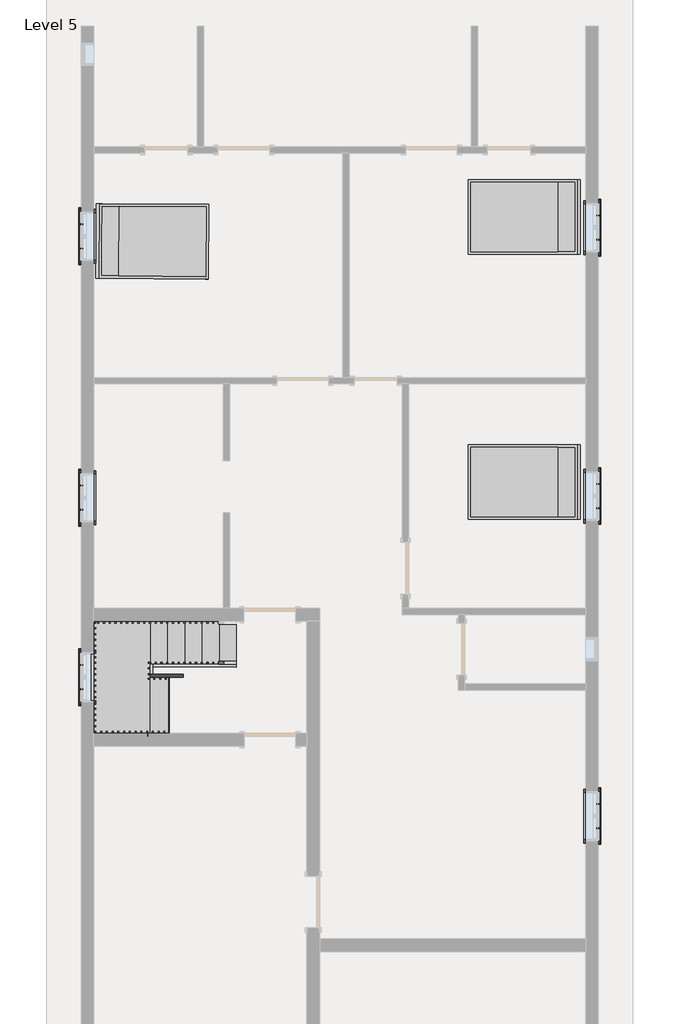
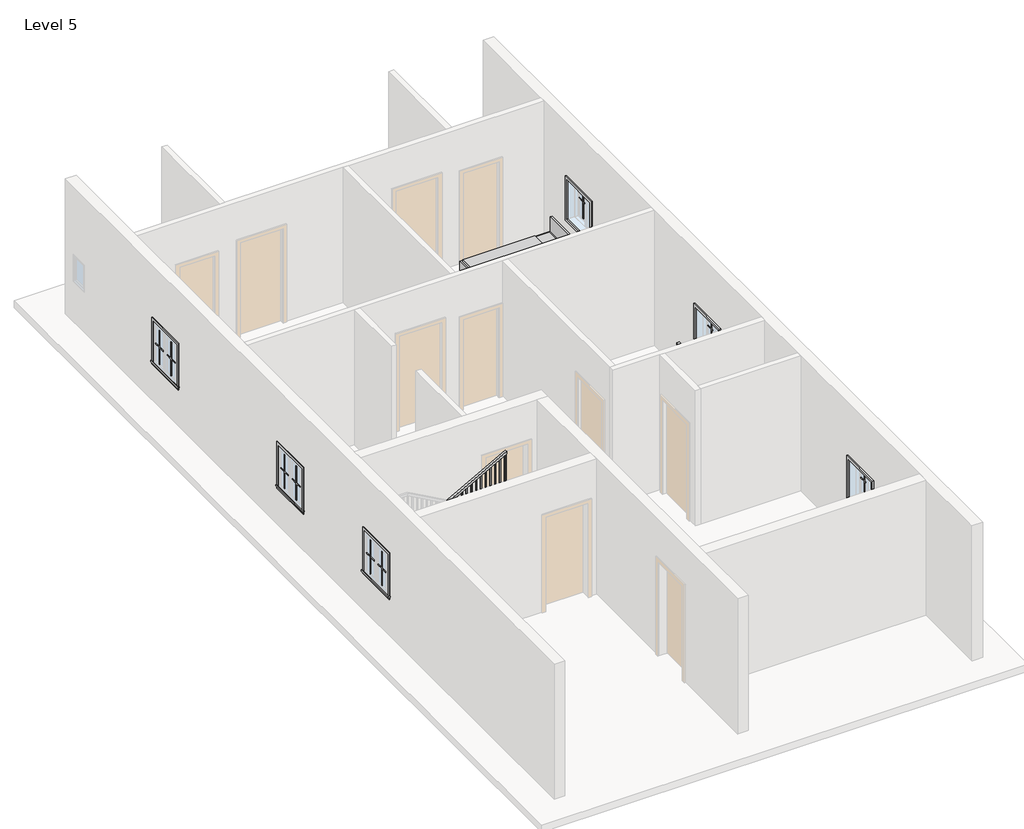
# One storey, part 3 of 3: 24 proxies, 6 members, 3 furniture elements, 1 railing, 1 stair flight.
"""IFC4 building model written with IfcOpenShell, lengths in millimetres."""

from ifc_helpers import new_model, si_unit, frame, origin, place, context, project, spatial, polyline, outline, extrude, faceted_brep, transform, mapped, element, save
from components import muntin_pattern_2x2_muntin_pattern_2x2_b3fe6957, muntin_pattern_2x2_muntin_pattern_2x2_3e0ecaf2, trim_window_exterior_flat_with_sill_41619996, trim_window_interior_flat_picture_frame_51c85655, bed_17739_bed_17739_15c61121, stair_flight_99d63151

model = new_model("IFC4")

# Units and contexts
model_context = context("Model", 3, world=origin())
ifc_project = project(units=[si_unit("LENGTHUNIT", "METRE", prefix="MILLI")], contexts=[model_context])

# Site, building, storey
site = spatial("IfcSite", under=ifc_project)
building = spatial("IfcBuilding", under=site)
storey = spatial("IfcBuildingStorey", under=building, Name="Level 5", Elevation=9601.2)

# Proxies
placement = place(None, origin())
muntin_pattern_2x2_muntin_pattern_2x2_shape = muntin_pattern_2x2_muntin_pattern_2x2_b3fe6957(model_context)
element("IfcBuildingElementProxy", 1, Name="Muntin Pattern_2x2 : Muntin Pattern_2x2", ObjectType="Muntin Pattern_2x2 : Muntin Pattern_2x2", at=placement, inside=storey, context=model_context, shape_type="MappedRepresentation", body=[
    mapped(muntin_pattern_2x2_muntin_pattern_2x2_shape, transform((3307.2334916, 6850.4197267, 10585.45), x_axis=(0.0, -1.0, 0.0), y_axis=(1.0, 0.0, 0.0), z_axis=(0.0, 0.0, 1.0))),
])
element("IfcBuildingElementProxy", 2, Name="Muntin Pattern_2x2 : Muntin Pattern_2x2", ObjectType="Muntin Pattern_2x2 : Muntin Pattern_2x2", at=placement, inside=storey, context=model_context, shape_type="MappedRepresentation", body=[
    mapped(muntin_pattern_2x2_muntin_pattern_2x2_shape, transform((3307.2334916, 2106.9697267, 10585.45), x_axis=(0.0, -1.0, 0.0), y_axis=(1.0, 0.0, 0.0), z_axis=(0.0, 0.0, 1.0))),
])
element("IfcBuildingElementProxy", 3, Name="Muntin Pattern_2x2 : Muntin Pattern_2x2", ObjectType="Muntin Pattern_2x2 : Muntin Pattern_2x2", at=placement, inside=storey, context=model_context, shape_type="MappedRepresentation", body=[
    mapped(muntin_pattern_2x2_muntin_pattern_2x2_shape, transform((-5817.7165084, 6269.3947267, 10585.45), x_axis=(0.0, 1.0, 0.0), y_axis=(-1.0, 0.0, 0.0), z_axis=(0.0, 0.0, 1.0))),
])
element("IfcBuildingElementProxy", 4, Name="Muntin Pattern_2x2 : Muntin Pattern_2x2", ObjectType="Muntin Pattern_2x2 : Muntin Pattern_2x2", at=placement, inside=storey, context=model_context, shape_type="MappedRepresentation", body=[
    mapped(muntin_pattern_2x2_muntin_pattern_2x2_shape, transform((-5817.7165084, 1649.7697267, 10585.45), x_axis=(0.0, 1.0, 0.0), y_axis=(-1.0, 0.0, 0.0), z_axis=(0.0, 0.0, 1.0))),
])
element("IfcBuildingElementProxy", 5, Name="Muntin Pattern_2x2 : Muntin Pattern_2x2", ObjectType="Muntin Pattern_2x2 : Muntin Pattern_2x2", at=placement, inside=storey, context=model_context, shape_type="MappedRepresentation", body=[
    mapped(muntin_pattern_2x2_muntin_pattern_2x2_shape, transform((3307.2334916, -3547.7052733, 10585.45), x_axis=(0.0, -1.0, 0.0), y_axis=(1.0, 0.0, 0.0), z_axis=(0.0, 0.0, 1.0))),
])
element("IfcBuildingElementProxy", 6, Name="Muntin Pattern_2x2 : Muntin Pattern_2x2", ObjectType="Muntin Pattern_2x2 : Muntin Pattern_2x2", at=placement, inside=storey, context=model_context, shape_type="MappedRepresentation", body=[
    mapped(muntin_pattern_2x2_muntin_pattern_2x2_shape, transform((-5817.7165084, -1522.0552733, 10585.45), x_axis=(0.0, 1.0, 0.0), y_axis=(-1.0, 0.0, 0.0), z_axis=(0.0, 0.0, 1.0))),
])
muntin_pattern_2x2_muntin_pattern_2x2_2_shape = muntin_pattern_2x2_muntin_pattern_2x2_3e0ecaf2(model_context)
element("IfcBuildingElementProxy", 7, Name="Muntin Pattern_2x2 : Muntin Pattern_2x2", ObjectType="Muntin Pattern_2x2 : Muntin Pattern_2x2", at=placement, inside=storey, context=model_context, shape_type="MappedRepresentation", body=[
    mapped(muntin_pattern_2x2_muntin_pattern_2x2_2_shape, transform((3307.2334916, 6421.7947267, 10585.45), x_axis=(0.0, 1.0, 0.0), y_axis=(-1.0, 0.0, 0.0), z_axis=(0.0, 0.0, 1.0))),
])
element("IfcBuildingElementProxy", 8, Name="Muntin Pattern_2x2 : Muntin Pattern_2x2", ObjectType="Muntin Pattern_2x2 : Muntin Pattern_2x2", at=placement, inside=storey, context=model_context, shape_type="MappedRepresentation", body=[
    mapped(muntin_pattern_2x2_muntin_pattern_2x2_2_shape, transform((3307.2334916, 1678.3447267, 10585.45), x_axis=(0.0, 1.0, 0.0), y_axis=(-1.0, 0.0, 0.0), z_axis=(0.0, 0.0, 1.0))),
])
element("IfcBuildingElementProxy", 9, Name="Muntin Pattern_2x2 : Muntin Pattern_2x2", ObjectType="Muntin Pattern_2x2 : Muntin Pattern_2x2", at=placement, inside=storey, context=model_context, shape_type="MappedRepresentation", body=[
    mapped(muntin_pattern_2x2_muntin_pattern_2x2_2_shape, transform((-5817.7165084, 6698.0197267, 10585.45), x_axis=(0.0, -1.0, 0.0), y_axis=(1.0, 0.0, 0.0), z_axis=(0.0, 0.0, 1.0))),
])
element("IfcBuildingElementProxy", 10, Name="Muntin Pattern_2x2 : Muntin Pattern_2x2", ObjectType="Muntin Pattern_2x2 : Muntin Pattern_2x2", at=placement, inside=storey, context=model_context, shape_type="MappedRepresentation", body=[
    mapped(muntin_pattern_2x2_muntin_pattern_2x2_2_shape, transform((-5817.7165084, 2078.3947267, 10585.45), x_axis=(0.0, -1.0, 0.0), y_axis=(1.0, 0.0, 0.0), z_axis=(0.0, 0.0, 1.0))),
])
element("IfcBuildingElementProxy", 11, Name="Muntin Pattern_2x2 : Muntin Pattern_2x2", ObjectType="Muntin Pattern_2x2 : Muntin Pattern_2x2", at=placement, inside=storey, context=model_context, shape_type="MappedRepresentation", body=[
    mapped(muntin_pattern_2x2_muntin_pattern_2x2_2_shape, transform((3307.2334916, -3976.3302733, 10585.45), x_axis=(0.0, 1.0, 0.0), y_axis=(-1.0, 0.0, 0.0), z_axis=(0.0, 0.0, 1.0))),
])
element("IfcBuildingElementProxy", 12, Name="Muntin Pattern_2x2 : Muntin Pattern_2x2", ObjectType="Muntin Pattern_2x2 : Muntin Pattern_2x2", at=placement, inside=storey, context=model_context, shape_type="MappedRepresentation", body=[
    mapped(muntin_pattern_2x2_muntin_pattern_2x2_2_shape, transform((-5817.7165084, -1093.4302733, 10585.45), x_axis=(0.0, -1.0, 0.0), y_axis=(1.0, 0.0, 0.0), z_axis=(0.0, 0.0, 1.0))),
])
trim_window_exterior_flat_with_sill_shape = trim_window_exterior_flat_with_sill_41619996(model_context)
element("IfcBuildingElementProxy", 13, Name="Trim-Window-Exterior-Flat : with Sill", ObjectType="Trim-Window-Exterior-Flat : with Sill", at=placement, inside=storey, context=model_context, shape_type="MappedRepresentation", body=[
    mapped(trim_window_exterior_flat_with_sill_shape, transform((3316.7584916, 6636.1072267, 11430.0), x_axis=(0.0, 1.0, 0.0), y_axis=(0.0, 0.0, 1.0), z_axis=(1.0, 0.0, 0.0))),
])
element("IfcBuildingElementProxy", 14, Name="Trim-Window-Exterior-Flat : with Sill", ObjectType="Trim-Window-Exterior-Flat : with Sill", at=placement, inside=storey, context=model_context, shape_type="MappedRepresentation", body=[
    mapped(trim_window_exterior_flat_with_sill_shape, transform((3316.7584916, 1892.6572267, 11430.0), x_axis=(0.0, 1.0, 0.0), y_axis=(0.0, 0.0, 1.0), z_axis=(1.0, 0.0, 0.0))),
])
element("IfcBuildingElementProxy", 15, Name="Trim-Window-Exterior-Flat : with Sill", ObjectType="Trim-Window-Exterior-Flat : with Sill", at=placement, inside=storey, context=model_context, shape_type="MappedRepresentation", body=[
    mapped(trim_window_exterior_flat_with_sill_shape, transform((-5827.2415084, 6483.7072267, 11430.0), x_axis=(0.0, -1.0, 0.0), y_axis=(0.0, 0.0, 1.0), z_axis=(-1.0, 0.0, 0.0))),
])
element("IfcBuildingElementProxy", 16, Name="Trim-Window-Exterior-Flat : with Sill", ObjectType="Trim-Window-Exterior-Flat : with Sill", at=placement, inside=storey, context=model_context, shape_type="MappedRepresentation", body=[
    mapped(trim_window_exterior_flat_with_sill_shape, transform((-5827.2415084, 1864.0822267, 11430.0), x_axis=(0.0, -1.0, 0.0), y_axis=(0.0, 0.0, 1.0), z_axis=(-1.0, 0.0, 0.0))),
])
element("IfcBuildingElementProxy", 17, Name="Trim-Window-Exterior-Flat : with Sill", ObjectType="Trim-Window-Exterior-Flat : with Sill", at=placement, inside=storey, context=model_context, shape_type="MappedRepresentation", body=[
    mapped(trim_window_exterior_flat_with_sill_shape, transform((3316.7584916, -3762.0177733, 11430.0), x_axis=(0.0, 1.0, 0.0), y_axis=(0.0, 0.0, 1.0), z_axis=(1.0, 0.0, 0.0))),
])
element("IfcBuildingElementProxy", 18, Name="Trim-Window-Exterior-Flat : with Sill", ObjectType="Trim-Window-Exterior-Flat : with Sill", at=placement, inside=storey, context=model_context, shape_type="MappedRepresentation", body=[
    mapped(trim_window_exterior_flat_with_sill_shape, transform((-5827.2415084, -1307.7427733, 11430.0), x_axis=(0.0, -1.0, 0.0), y_axis=(0.0, 0.0, 1.0), z_axis=(-1.0, 0.0, 0.0))),
])
trim_window_interior_flat_picture_frame_shape = trim_window_interior_flat_picture_frame_51c85655(model_context)
element("IfcBuildingElementProxy", 19, Name="Trim-Window-Interior-Flat : Picture Frame", ObjectType="Trim-Window-Interior-Flat : Picture Frame", at=placement, inside=storey, context=model_context, shape_type="MappedRepresentation", body=[
    mapped(trim_window_interior_flat_picture_frame_shape, transform((3088.1584916, 6636.1072267, 11430.0), x_axis=(0.0, -1.0, 0.0), y_axis=(0.0, 0.0, 1.0), z_axis=(-1.0, 0.0, 0.0))),
])
element("IfcBuildingElementProxy", 20, Name="Trim-Window-Interior-Flat : Picture Frame", ObjectType="Trim-Window-Interior-Flat : Picture Frame", at=placement, inside=storey, context=model_context, shape_type="MappedRepresentation", body=[
    mapped(trim_window_interior_flat_picture_frame_shape, transform((3088.1584916, 1892.6572267, 11430.0), x_axis=(0.0, -1.0, 0.0), y_axis=(0.0, 0.0, 1.0), z_axis=(-1.0, 0.0, 0.0))),
])
element("IfcBuildingElementProxy", 21, Name="Trim-Window-Interior-Flat : Picture Frame", ObjectType="Trim-Window-Interior-Flat : Picture Frame", at=placement, inside=storey, context=model_context, shape_type="MappedRepresentation", body=[
    mapped(trim_window_interior_flat_picture_frame_shape, transform((-5598.6415084, 6483.7072267, 11430.0), x_axis=(0.0, 1.0, 0.0), y_axis=(0.0, 0.0, 1.0), z_axis=(1.0, 0.0, 0.0))),
])
element("IfcBuildingElementProxy", 22, Name="Trim-Window-Interior-Flat : Picture Frame", ObjectType="Trim-Window-Interior-Flat : Picture Frame", at=placement, inside=storey, context=model_context, shape_type="MappedRepresentation", body=[
    mapped(trim_window_interior_flat_picture_frame_shape, transform((-5598.6415084, 1864.0822267, 11430.0), x_axis=(0.0, 1.0, 0.0), y_axis=(0.0, 0.0, 1.0), z_axis=(1.0, 0.0, 0.0))),
])
element("IfcBuildingElementProxy", 23, Name="Trim-Window-Interior-Flat : Picture Frame", ObjectType="Trim-Window-Interior-Flat : Picture Frame", at=placement, inside=storey, context=model_context, shape_type="MappedRepresentation", body=[
    mapped(trim_window_interior_flat_picture_frame_shape, transform((3088.1584916, -3762.0177733, 11430.0), x_axis=(0.0, -1.0, 0.0), y_axis=(0.0, 0.0, 1.0), z_axis=(-1.0, 0.0, 0.0))),
])
element("IfcBuildingElementProxy", 24, Name="Trim-Window-Interior-Flat : Picture Frame", ObjectType="Trim-Window-Interior-Flat : Picture Frame", at=placement, inside=storey, context=model_context, shape_type="MappedRepresentation", body=[
    mapped(trim_window_interior_flat_picture_frame_shape, transform((-5598.6415084, -1307.7427733, 11430.0), x_axis=(0.0, 1.0, 0.0), y_axis=(0.0, 0.0, 1.0), z_axis=(1.0, 0.0, 0.0))),
])

# Furniture
bed_17739_bed_17739_shape = bed_17739_bed_17739_15c61121(model_context)
element("IfcFurniture", 25, ObjectType="Bed_17739 : Bed_17739", at=placement, inside=storey, context=model_context, shape_type="MappedRepresentation", body=[
    mapped(bed_17739_bed_17739_shape, transform((-4543.6279345, 6394.2844586, 9601.2), x_axis=(0.007593038844487308, 0.9999711724650396, 0.0), y_axis=(-0.9999711724650396, 0.007593038844487308, 0.0), z_axis=(0.0, 0.0, 1.0))),
])
element("IfcFurniture", 26, ObjectType="Bed_17739 : Bed_17739", at=placement, inside=storey, context=model_context, shape_type="MappedRepresentation", body=[
    mapped(bed_17739_bed_17739_shape, transform((1983.2584916, 6826.6072267, 9601.2), x_axis=(0.0, -1.0, 0.0), y_axis=(1.0, 0.0, 0.0), z_axis=(0.0, 0.0, 1.0))),
])
element("IfcFurniture", 27, ObjectType="Bed_17739 : Bed_17739", at=placement, inside=storey, context=model_context, shape_type="MappedRepresentation", body=[
    mapped(bed_17739_bed_17739_shape, transform((1983.2584916, 2140.3072267, 9601.2), x_axis=(0.0, -1.0, 0.0), y_axis=(1.0, 0.0, 0.0), z_axis=(0.0, 0.0, 1.0))),
])

# Members
element("IfcMember", 28, ObjectType="Stringer - 2\" Width", at=placement, inside=storey, context=model_context, shape_type="SweptSolid", body=[
    extrude(outline(polyline([(9601.2, -3084.0415084), (9808.7983948, -3084.0415084), (10627.2428392, -4557.2415084), (10278.5641651, -4557.2415084), (9601.2, -3337.9860112), (9601.2, -3084.0415084)])), frame((0.0, -1127.4758739, 0.0), z_axis=(0.0, 1.0, 0.0), x_axis=(0.0, 0.0, 1.0)), (0.0, 0.0, 1.0), 50.8),
])
element("IfcMember", 29, ObjectType="Stringer - 2\" Width", at=placement, inside=storey, context=model_context, shape_type="SweptSolid", body=[
    extrude(outline(polyline([(-4608.0415084, -1076.6758739), (-4557.2415084, -1076.6758739), (-4557.2415084, -1256.9427733), (-4608.0415084, -1256.9427733), (-4608.0415084, -1076.6758739)])), frame((0.0, 0.0, 10388.6), z_axis=(0.0, 0.0, 1.0), x_axis=(1.0, 0.0, 0.0)), (0.0, 0.0, 1.0), 304.8),
])
element("IfcMember", 30, ObjectType="Stringer - 2\" Width", at=placement, inside=storey, context=model_context, shape_type="SweptSolid", body=[
    extrude(outline(polyline([(10824.7983948, -4608.0415084), (10476.1197207, -4608.0415084), (11322.7863873, -3084.0415084), (11671.4650614, -3084.0415084), (10824.7983948, -4608.0415084)])), frame((0.0, -1307.7427733, 0.0), z_axis=(0.0, 1.0, 0.0), x_axis=(0.0, 0.0, 1.0)), (0.0, 0.0, 1.0), 50.8),
])
element("IfcMember", 31, ObjectType="Stringer - 2\" Width", at=placement, inside=storey, context=model_context, shape_type="SweptSolid", body=[
    extrude(outline(polyline([(9601.2, -3084.0415084), (9808.7983948, -3084.0415084), (10693.4, -4676.3243978), (10693.4, -5303.9460112), (9601.2, -3337.9860112), (9601.2, -3084.0415084)])), frame((0.0, -317.1427733, 0.0), z_axis=(0.0, 1.0, 0.0), x_axis=(0.0, 0.0, 1.0)), (0.0, 0.0, 1.0), 50.8),
])
element("IfcMember", 32, ObjectType="Stringer - 2\" Width", at=placement, inside=storey, context=model_context, shape_type="SweptSolid", body=[
    extrude(outline(polyline([(-5649.4415084, -266.3427733), (-5598.6415084, -266.3427733), (-5598.6415084, -2298.3427733), (-5649.4415084, -2298.3427733), (-5649.4415084, -266.3427733)])), frame((0.0, 0.0, 10388.6), z_axis=(0.0, 0.0, 1.0), x_axis=(1.0, 0.0, 0.0)), (0.0, 0.0, 1.0), 304.8),
])
element("IfcMember", 33, ObjectType="Stringer - 2\" Width", at=placement, inside=storey, context=model_context, shape_type="SweptSolid", body=[
    extrude(outline(polyline([(10388.6, -4765.5770056), (11322.7863873, -3084.0415084), (11671.4650614, -3084.0415084), (10388.6, -5393.198619), (10388.6, -4765.5770056)])), frame((0.0, -2349.1427733, 0.0), z_axis=(0.0, 1.0, 0.0), x_axis=(0.0, 0.0, 1.0)), (0.0, 0.0, 1.0), 50.8),
])

# Railing
element("IfcRailing", 34, ObjectType="Handrail - Rectangular", at=placement, inside=storey, context=model_context, shape_type="SolidModel", body=[
    faceted_brep([(-3084.0415084, -1076.6758739, 10684.9333333), (-3084.0415084, -1076.6758739, 10626.820221), (-3084.0415084, -1025.8758739, 10626.820221), (-3084.0415084, -1025.8758739, 10684.9333333), (-4531.8415084, -1076.6758739, 11489.2666667), (-4582.6415084, -1076.6758739, 11459.3757765), (-4582.6415084, -1025.8758739, 11459.3757765), (-4531.8415084, -1025.8758739, 11489.2666667), (-4531.8415084, -1076.6758739, 11531.6), (-4582.6415084, -1076.6758739, 11480.8), (-4582.6415084, -1025.8758739, 11480.8), (-4531.8415084, -1025.8758739, 11531.6), (-4608.0415084, -1076.6758739, 11531.6), (-4608.0415084, -1076.6758739, 11480.8), (-4658.8415084, -1025.8758739, 11480.8), (-4658.8415084, -1025.8758739, 11531.6), (-4608.0415084, -1152.8758739, 11531.6), (-4608.0415084, -1152.8758739, 11480.8), (-4658.8415084, -1152.8758739, 11480.8), (-4658.8415084, -1152.8758739, 11531.6), (-4608.0415084, -1231.5427733, 11531.6), (-4608.0415084, -1282.3427733, 11480.8), (-4658.8415084, -1282.3427733, 11480.8), (-4658.8415084, -1231.5427733, 11531.6), (-4608.0415084, -1231.5427733, 11743.2666667), (-4608.0415084, -1282.3427733, 11692.4666667), (-4658.8415084, -1282.3427733, 11692.4666667), (-4658.8415084, -1231.5427733, 11743.2666667), (-4608.0415084, -1307.7427733, 11743.2666667), (-4608.0415084, -1307.7427733, 11692.4666667), (-4658.8415084, -1358.5427733, 11692.4666667), (-4658.8415084, -1358.5427733, 11743.2666667), (-4531.8415084, -1307.7427733, 11743.2666667), (-4518.6779062, -1307.7427733, 11692.4666667), (-4518.6779062, -1358.5427733, 11692.4666667), (-4531.8415084, -1358.5427733, 11743.2666667), (-3084.0415084, -1307.7427733, 12547.6), (-3084.0415084, -1358.5427733, 12547.6), (-3084.0415084, -1358.5427733, 12489.4868876), (-3084.0415084, -1307.7427733, 12489.4868876)], [[[0, 1, 2, 3]], [[1, 0, 4, 5]], [[2, 1, 5, 6]], [[3, 2, 6, 7]], [[0, 3, 7, 4]], [[5, 4, 8, 9]], [[6, 5, 9, 10]], [[7, 6, 10, 11]], [[4, 7, 11, 8]], [[9, 8, 12, 13]], [[10, 9, 13, 14]], [[11, 10, 14, 15]], [[8, 11, 15, 12]], [[13, 12, 16, 17]], [[14, 13, 17, 18]], [[15, 14, 18, 19]], [[12, 15, 19, 16]], [[17, 16, 20, 21]], [[18, 17, 21, 22]], [[19, 18, 22, 23]], [[16, 19, 23, 20]], [[21, 20, 24, 25]], [[22, 21, 25, 26]], [[23, 22, 26, 27]], [[20, 23, 27, 24]], [[25, 24, 28, 29]], [[26, 25, 29, 30]], [[27, 26, 30, 31]], [[24, 27, 31, 28]], [[29, 28, 32, 33]], [[30, 29, 33, 34]], [[31, 30, 34, 35]], [[28, 31, 35, 32]], [[36, 37, 38, 39]], [[33, 32, 36, 39]], [[34, 33, 39, 38]], [[35, 34, 38, 37]], [[32, 35, 37, 36]]]),
    extrude(outline(polyline([(12470.0841099, -3118.9665084), (11463.8666667, -3118.9665084), (11463.8666667, -3099.9165084), (12480.6674432, -3099.9165084), (12470.0841099, -3118.9665084)])), frame((0.0, -1342.6677733, 0.0), z_axis=(0.0, 1.0, 0.0), x_axis=(0.0, 0.0, 1.0)), (0.0, 0.0, 1.0), 19.05),
    extrude(outline(polyline([(12413.6396654, -3220.5665084), (11463.8666667, -3220.5665084), (11463.8666667, -3201.5165084), (12424.2229988, -3201.5165084), (12413.6396654, -3220.5665084)])), frame((0.0, -1342.6677733, 0.0), z_axis=(0.0, 1.0, 0.0), x_axis=(0.0, 0.0, 1.0)), (0.0, 0.0, 1.0), 19.05),
    extrude(outline(polyline([(12357.195221, -3322.1665084), (11463.8666667, -3322.1665084), (11463.8666667, -3303.1165084), (12367.7785543, -3303.1165084), (12357.195221, -3322.1665084)])), frame((0.0, -1342.6677733, 0.0), z_axis=(0.0, 1.0, 0.0), x_axis=(0.0, 0.0, 1.0)), (0.0, 0.0, 1.0), 19.05),
    extrude(outline(polyline([(12300.7507765, -3423.7665084), (11294.5333333, -3423.7665084), (11294.5333333, -3404.7165084), (12311.3341099, -3404.7165084), (12300.7507765, -3423.7665084)])), frame((0.0, -1342.6677733, 0.0), z_axis=(0.0, 1.0, 0.0), x_axis=(0.0, 0.0, 1.0)), (0.0, 0.0, 1.0), 19.05),
    extrude(outline(polyline([(12244.3063321, -3525.3665084), (11294.5333333, -3525.3665084), (11294.5333333, -3506.3165084), (12254.8896654, -3506.3165084), (12244.3063321, -3525.3665084)])), frame((0.0, -1342.6677733, 0.0), z_axis=(0.0, 1.0, 0.0), x_axis=(0.0, 0.0, 1.0)), (0.0, 0.0, 1.0), 19.05),
    extrude(outline(polyline([(12187.8618876, -3626.9665084), (11294.5333333, -3626.9665084), (11294.5333333, -3607.9165084), (12198.445221, -3607.9165084), (12187.8618876, -3626.9665084)])), frame((0.0, -1342.6677733, 0.0), z_axis=(0.0, 1.0, 0.0), x_axis=(0.0, 0.0, 1.0)), (0.0, 0.0, 1.0), 19.05),
    extrude(outline(polyline([(12131.4174432, -3728.5665084), (11125.2, -3728.5665084), (11125.2, -3709.5165084), (12142.0007765, -3709.5165084), (12131.4174432, -3728.5665084)])), frame((0.0, -1342.6677733, 0.0), z_axis=(0.0, 1.0, 0.0), x_axis=(0.0, 0.0, 1.0)), (0.0, 0.0, 1.0), 19.05),
    extrude(outline(polyline([(12074.9729988, -3830.1665084), (11125.2, -3830.1665084), (11125.2, -3811.1165084), (12085.5563321, -3811.1165084), (12074.9729988, -3830.1665084)])), frame((0.0, -1342.6677733, 0.0), z_axis=(0.0, 1.0, 0.0), x_axis=(0.0, 0.0, 1.0)), (0.0, 0.0, 1.0), 19.05),
    extrude(outline(polyline([(12018.5285543, -3931.7665084), (11125.2, -3931.7665084), (11125.2, -3912.7165084), (12029.1118876, -3912.7165084), (12018.5285543, -3931.7665084)])), frame((0.0, -1342.6677733, 0.0), z_axis=(0.0, 1.0, 0.0), x_axis=(0.0, 0.0, 1.0)), (0.0, 0.0, 1.0), 19.05),
    extrude(outline(polyline([(11962.0841099, -4033.3665084), (10955.8666667, -4033.3665084), (10955.8666667, -4014.3165084), (11972.6674432, -4014.3165084), (11962.0841099, -4033.3665084)])), frame((0.0, -1342.6677733, 0.0), z_axis=(0.0, 1.0, 0.0), x_axis=(0.0, 0.0, 1.0)), (0.0, 0.0, 1.0), 19.05),
    extrude(outline(polyline([(11905.6396654, -4134.9665084), (10955.8666667, -4134.9665084), (10955.8666667, -4115.9165084), (11916.2229988, -4115.9165084), (11905.6396654, -4134.9665084)])), frame((0.0, -1342.6677733, 0.0), z_axis=(0.0, 1.0, 0.0), x_axis=(0.0, 0.0, 1.0)), (0.0, 0.0, 1.0), 19.05),
    extrude(outline(polyline([(11849.195221, -4236.5665084), (10955.8666667, -4236.5665084), (10955.8666667, -4217.5165084), (11859.7785543, -4217.5165084), (11849.195221, -4236.5665084)])), frame((0.0, -1342.6677733, 0.0), z_axis=(0.0, 1.0, 0.0), x_axis=(0.0, 0.0, 1.0)), (0.0, 0.0, 1.0), 19.05),
    extrude(outline(polyline([(11792.7507765, -4338.1665084), (10786.5333333, -4338.1665084), (10786.5333333, -4319.1165084), (11803.3341099, -4319.1165084), (11792.7507765, -4338.1665084)])), frame((0.0, -1342.6677733, 0.0), z_axis=(0.0, 1.0, 0.0), x_axis=(0.0, 0.0, 1.0)), (0.0, 0.0, 1.0), 19.05),
    extrude(outline(polyline([(11736.3063321, -4439.7665084), (10786.5333333, -4439.7665084), (10786.5333333, -4420.7165084), (11746.8896654, -4420.7165084), (11736.3063321, -4439.7665084)])), frame((0.0, -1342.6677733, 0.0), z_axis=(0.0, 1.0, 0.0), x_axis=(0.0, 0.0, 1.0)), (0.0, 0.0, 1.0), 19.05),
    extrude(outline(polyline([(11679.8618876, -4541.3665084), (10786.5333333, -4541.3665084), (10786.5333333, -4522.3165084), (11690.445221, -4522.3165084), (11679.8618876, -4541.3665084)])), frame((0.0, -1342.6677733, 0.0), z_axis=(0.0, 1.0, 0.0), x_axis=(0.0, 0.0, 1.0)), (0.0, 0.0, 1.0), 19.05),
    extrude(outline(polyline([(-4623.9165084, -1244.9508739), (-4623.9165084, -1264.0008739), (-4642.9665084, -1264.0008739), (-4642.9665084, -1244.9508739), (-4623.9165084, -1244.9508739)])), frame((0.0, 0.0, 10617.2), z_axis=(0.0, 0.0, 1.0), x_axis=(1.0, 0.0, 0.0)), (0.0, 0.0, 1.0), 1075.2666667),
    extrude(outline(polyline([(-4623.9165084, -1143.3508739), (-4623.9165084, -1162.4008739), (-4642.9665084, -1162.4008739), (-4642.9665084, -1143.3508739), (-4623.9165084, -1143.3508739)])), frame((0.0, 0.0, 10617.2), z_axis=(0.0, 0.0, 1.0), x_axis=(1.0, 0.0, 0.0)), (0.0, 0.0, 1.0), 863.6),
    extrude(outline(polyline([(-4598.5165084, -1060.8008739), (-4617.5665084, -1060.8008739), (-4617.5665084, -1041.7508739), (-4598.5165084, -1041.7508739), (-4598.5165084, -1060.8008739)])), frame((0.0, 0.0, 10617.2), z_axis=(0.0, 0.0, 1.0), x_axis=(1.0, 0.0, 0.0)), (0.0, 0.0, 1.0), 863.6),
    extrude(outline(polyline([(11422.3341099, -4515.9665084), (10447.8666667, -4515.9665084), (10447.8666667, -4496.9165084), (11411.7507765, -4496.9165084), (11422.3341099, -4515.9665084)])), frame((0.0, -1060.8008739, 0.0), z_axis=(0.0, 1.0, 0.0), x_axis=(0.0, 0.0, 1.0)), (0.0, 0.0, 1.0), 19.05),
    extrude(outline(polyline([(11365.8896654, -4414.3665084), (10447.8666667, -4414.3665084), (10447.8666667, -4395.3165084), (11355.3063321, -4395.3165084), (11365.8896654, -4414.3665084)])), frame((0.0, -1060.8008739, 0.0), z_axis=(0.0, 1.0, 0.0), x_axis=(0.0, 0.0, 1.0)), (0.0, 0.0, 1.0), 19.05),
    extrude(outline(polyline([(11309.445221, -4312.7665084), (10447.8666667, -4312.7665084), (10447.8666667, -4293.7165084), (11298.8618876, -4293.7165084), (11309.445221, -4312.7665084)])), frame((0.0, -1060.8008739, 0.0), z_axis=(0.0, 1.0, 0.0), x_axis=(0.0, 0.0, 1.0)), (0.0, 0.0, 1.0), 19.05),
    extrude(outline(polyline([(11253.0007765, -4211.1665084), (10278.5333333, -4211.1665084), (10278.5333333, -4192.1165084), (11242.4174432, -4192.1165084), (11253.0007765, -4211.1665084)])), frame((0.0, -1060.8008739, 0.0), z_axis=(0.0, 1.0, 0.0), x_axis=(0.0, 0.0, 1.0)), (0.0, 0.0, 1.0), 19.05),
    extrude(outline(polyline([(11196.5563321, -4109.5665084), (10278.5333333, -4109.5665084), (10278.5333333, -4090.5165084), (11185.9729988, -4090.5165084), (11196.5563321, -4109.5665084)])), frame((0.0, -1060.8008739, 0.0), z_axis=(0.0, 1.0, 0.0), x_axis=(0.0, 0.0, 1.0)), (0.0, 0.0, 1.0), 19.05),
    extrude(outline(polyline([(11140.1118876, -4007.9665084), (10278.5333333, -4007.9665084), (10278.5333333, -3988.9165084), (11129.5285543, -3988.9165084), (11140.1118876, -4007.9665084)])), frame((0.0, -1060.8008739, 0.0), z_axis=(0.0, 1.0, 0.0), x_axis=(0.0, 0.0, 1.0)), (0.0, 0.0, 1.0), 19.05),
    extrude(outline(polyline([(11083.6674432, -3906.3665084), (10109.2, -3906.3665084), (10109.2, -3887.3165084), (11073.0841099, -3887.3165084), (11083.6674432, -3906.3665084)])), frame((0.0, -1060.8008739, 0.0), z_axis=(0.0, 1.0, 0.0), x_axis=(0.0, 0.0, 1.0)), (0.0, 0.0, 1.0), 19.05),
    extrude(outline(polyline([(11027.2229988, -3804.7665084), (10109.2, -3804.7665084), (10109.2, -3785.7165084), (11016.6396654, -3785.7165084), (11027.2229988, -3804.7665084)])), frame((0.0, -1060.8008739, 0.0), z_axis=(0.0, 1.0, 0.0), x_axis=(0.0, 0.0, 1.0)), (0.0, 0.0, 1.0), 19.05),
    extrude(outline(polyline([(10970.7785543, -3703.1665084), (10109.2, -3703.1665084), (10109.2, -3684.1165084), (10960.195221, -3684.1165084), (10970.7785543, -3703.1665084)])), frame((0.0, -1060.8008739, 0.0), z_axis=(0.0, 1.0, 0.0), x_axis=(0.0, 0.0, 1.0)), (0.0, 0.0, 1.0), 19.05),
    extrude(outline(polyline([(10914.3341099, -3601.5665084), (9939.8666667, -3601.5665084), (9939.8666667, -3582.5165084), (10903.7507765, -3582.5165084), (10914.3341099, -3601.5665084)])), frame((0.0, -1060.8008739, 0.0), z_axis=(0.0, 1.0, 0.0), x_axis=(0.0, 0.0, 1.0)), (0.0, 0.0, 1.0), 19.05),
    extrude(outline(polyline([(10857.8896654, -3499.9665084), (9939.8666667, -3499.9665084), (9939.8666667, -3480.9165084), (10847.3063321, -3480.9165084), (10857.8896654, -3499.9665084)])), frame((0.0, -1060.8008739, 0.0), z_axis=(0.0, 1.0, 0.0), x_axis=(0.0, 0.0, 1.0)), (0.0, 0.0, 1.0), 19.05),
    extrude(outline(polyline([(10801.445221, -3398.3665084), (9939.8666667, -3398.3665084), (9939.8666667, -3379.3165084), (10790.8618876, -3379.3165084), (10801.445221, -3398.3665084)])), frame((0.0, -1060.8008739, 0.0), z_axis=(0.0, 1.0, 0.0), x_axis=(0.0, 0.0, 1.0)), (0.0, 0.0, 1.0), 19.05),
    extrude(outline(polyline([(10745.0007765, -3296.7665084), (9770.5333333, -3296.7665084), (9770.5333333, -3277.7165084), (10734.4174432, -3277.7165084), (10745.0007765, -3296.7665084)])), frame((0.0, -1060.8008739, 0.0), z_axis=(0.0, 1.0, 0.0), x_axis=(0.0, 0.0, 1.0)), (0.0, 0.0, 1.0), 19.05),
    extrude(outline(polyline([(10688.5563321, -3195.1665084), (9770.5333333, -3195.1665084), (9770.5333333, -3176.1165084), (10677.9729988, -3176.1165084), (10688.5563321, -3195.1665084)])), frame((0.0, -1060.8008739, 0.0), z_axis=(0.0, 1.0, 0.0), x_axis=(0.0, 0.0, 1.0)), (0.0, 0.0, 1.0), 19.05),
    extrude(outline(polyline([(-4623.9165084, -1323.6177733), (-4623.9165084, -1342.6677733), (-4642.9665084, -1342.6677733), (-4642.9665084, -1323.6177733), (-4623.9165084, -1323.6177733)])), frame((0.0, 0.0, 10617.2), z_axis=(0.0, 0.0, 1.0), x_axis=(1.0, 0.0, 0.0)), (0.0, 0.0, 1.0), 1075.2666667),
    extrude(outline(polyline([(-4623.9165084, -1060.8008739), (-4642.9665084, -1060.8008739), (-4642.9665084, -1041.7508739), (-4623.9165084, -1041.7508739), (-4623.9165084, -1060.8008739)])), frame((0.0, 0.0, 10617.2), z_axis=(0.0, 0.0, 1.0), x_axis=(1.0, 0.0, 0.0)), (0.0, 0.0, 1.0), 863.6),
    extrude(outline(polyline([(12478.9035543, -3103.0915084), (11463.8666667, -3103.0915084), (11463.8666667, -3084.0415084), (12489.4868876, -3084.0415084), (12478.9035543, -3103.0915084)])), frame((0.0, -1342.6677733, 0.0), z_axis=(0.0, 1.0, 0.0), x_axis=(0.0, 0.0, 1.0)), (0.0, 0.0, 1.0), 19.05),
    extrude(outline(polyline([(10637.4035543, -3103.0915084), (9770.5333333, -3103.0915084), (9770.5333333, -3084.0415084), (10626.820221, -3084.0415084), (10637.4035543, -3103.0915084)])), frame((0.0, -1060.8008739, 0.0), z_axis=(0.0, 1.0, 0.0), x_axis=(0.0, 0.0, 1.0)), (0.0, 0.0, 1.0), 19.05),
])

# Stair flight
stair_flight_shape = stair_flight_99d63151(model_context)
element("IfcStairFlight", 35, ObjectType="2\" Tread 1\" Nosing 1/4\" Riser", at=placement, inside=storey, context=model_context, shape_type="MappedRepresentation", body=[
    mapped(stair_flight_shape, transform((0.0, 0.0, 0.0), x_axis=(1.0, 0.0, 0.0), y_axis=(0.0, 1.0, 0.0), z_axis=(0.0, 0.0, 1.0))),
])

save(model, "model.ifc")

# Revit data of these elements
# Type "Muntin Pattern_2x2 : Muntin Pattern_2x2"
#   Width [instance default] = 4' - 0"
#   Thickness = 0' - 0 1/2"
#   Height [instance default] = 4' - 0"
#   Distance = 0' - 0 3/4"
#   Interior Material [instance default] = none
#   Exterior Material [instance default] = none
#   Default Elevation = 0
# Type "Trim-Window-Exterior-Flat : with Sill"
#   Trim Width = 0' - 2 1/4"
#   Trim Thickness_Picture Frame = 0' - 1 1/4"
#   Trim Thickness_with Sill = 0' - 0 3/4"
#   Sill Thickness = 0' - 1 1/4"
#   Opening Width [instance default] = 2' - 0"
#   Opening Height [instance default] = 3' - 0"
#   Default Elevation = 4' - 0"
#   Sill = yes
#   Picture Frame = no
#   Trim Material [instance default] = none
# Type "Trim-Window-Interior-Flat : Picture Frame"
#   Trim Thickness_Picture Frame = 0' - 1 1/4"
#   Trim Width = 0' - 2 1/4"
#   Trim Thickness_with Sill = 0' - 0 3/4"
#   Sill Thickness = 0' - 1 1/4"
#   Opening Width [instance default] = 2' - 0"
#   Opening Height [instance default] = 3' - 0"
#   Default Elevation = 4' - 0"
#   Sill = no
#   Picture Frame = yes
#   Trim Material [instance default] = none
# Type "Bed_17739 : Bed_17739"
#   Default Elevation = 0
# Type "Handrail - Rectangular"
#   Assembly Code = "C2010400"
#   built-in parameter 1008612 = 0.0416667 (stored number, unit not read)
#   built-in parameter 1008611 = 0.0416667 (stored number, unit not read)
#   built-in parameter 1008609 = 0.333333 (stored number, unit not read)
#   built-in parameter 1008604 = 0.166667 (stored number, unit not read)
#   built-in parameter 1008603 = 0.166667 (stored number, unit not read)
#   Railing Height = 3' - 0"
#   built-in parameter 1008630 = 2
#   built-in parameter 1008610 = 2
#   built-in parameter 1008618 = Baluster - Square : 3/4"
# Elements 1, 2, 3, 4, 5, 6, 7, 8, 9, 10, 11, 12 (IfcBuildingElementProxy, "Muntin Pattern_2x2 : Muntin Pattern_2x2")
#   Width = 0' - 11 5/8"
#   Height = 2' - 6 1/2"
#   Interior Material = Wood - Stained
#   Exterior Material = Clad - White
#   Phase Created = New Construction
#   Materials on its faces: "Clad - White", "Wood - Stained"
# Elements 13, 14, 15, 16, 17, 18 (IfcBuildingElementProxy, "Trim-Window-Exterior-Flat : with Sill")
#   Opening Width = 2' - 10"
#   Opening Height = 3' - 0"
#   Trim Material = Clad - White
#   Phase Created = New Construction
#   Materials on its faces: "Clad - White"
# Elements 19, 20, 21, 22, 23, 24 (IfcBuildingElementProxy, "Trim-Window-Interior-Flat : Picture Frame")
#   Opening Width = 2' - 10"
#   Opening Height = 3' - 0"
#   Trim Material = Wood - Stained
#   Phase Created = New Construction
#   Materials on its faces: "Wood - Stained"
# Elements 25, 26, 27 (IfcFurniture, "Bed_17739 : Bed_17739")
#   Phase Created = New Construction
#   Materials on its faces: "legs", "sheets", "bed frame", "Blanket"
# Elements 28, 29, 30, 31, 32, 33 (IfcMember, "Stringer - 2\" Width")
#   Phase Created = New Construction
# Element 34 (IfcRailing, "Handrail - Rectangular")
#   Phase Created = New Construction
# Element 35 (IfcStairFlight, "2\" Tread 1\" Nosing 1/4\" Riser")
#   Phase Created = New Construction
# Materials
#   "Clad - White": class "Wood", colour RGB 242 242 238, transparency 0, Cost = 0
#   "Wood - Stained": class "Wood", colour RGB 224 178 126, transparency 0, Cost = 0
#   "legs": colour RGB 90 73 37, transparency 0, Cost = 0
#   "sheets": colour RGB 200 195 176, transparency 0, Cost = 0
#   "bed frame": colour RGB 90 73 37, transparency 0, Cost = 0
#   "Blanket": class "System", colour RGB 59 0 1, transparency 0, Cost = 0
